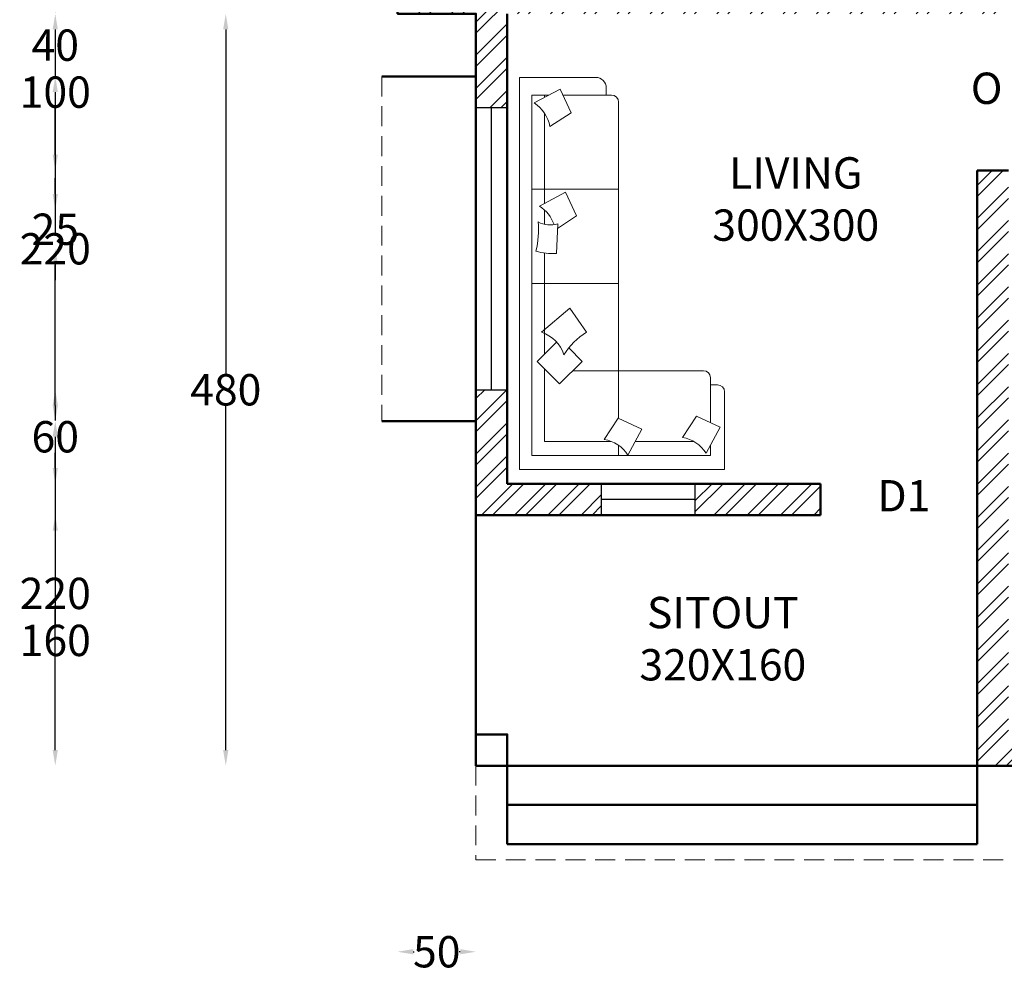
# Model space of a CAD drawing. Units: centimetres. Extents: x 10444 to 13814, y 8288 to 11191.
# Tile 2 of 9: x 10444 to 11072, y 9789 to 10397. Entities that reach past the tile are written whole.
import ezdxf

# ---------------------------------------------------------------- set-up
doc = ezdxf.new("R2010")
doc.units = ezdxf.units.CM
doc.header["$MEASUREMENT"] = 0
doc.linetypes.add('DASHED', pattern=[19.05, 12.7, -6.35])
for name, color, linetype, lineweight in [('A-ANNO-DIMS', 2, 'Continuous', 18), ('A-ANNO-TEXT', 7, 'Continuous', 25), ('A-AREA-IDEN', 3, 'Continuous', 25), ('A-FURN', 8, 'Continuous', 18), ('A-GLAZ', 4, 'Continuous', 25), ('A-ROOF-OVHD', 6, 'DASHED', 18), ('A-WALL', 7, 'Continuous', 50), ('A-WALL-PATT', 8, 'Continuous', 13)]:
    doc.layers.add(name, color=color, linetype=linetype, lineweight=lineweight)
doc.styles.get("Standard").update_dxf_attribs({"font": 'arial.ttf'})
doc.dimstyles.get("Standard").update_dxf_attribs({"dimtxt": 20, "dimasz": 10, "dimexe": 0.18, "dimexo": 0.0625, "dimgap": 0.09, "dimtad": 0, "dimtih": 1, "dimtoh": 1, "dimdec": 0, "dimzin": 0, "dimdsep": 46, "dimtxsty": 'Standard', "dimcen": 0.09, "dimse1": 1, "dimse2": 1, "dimadec": 0, "dimazin": 0, "dimtfac": 1, "dimtdec": 0, "dimtofl": 0, "dimtmove": 0, "dimatfit": 3, "dimfxl": 1, "dimtolj": 1, "dimtzin": 0, "dimarcsym": 0})

# ---------------------------------------------------------------- blocks, each defined once
blk = doc.blocks.new('s')
at = {"color": 0, "linetype": 'ByBlock'}
for p, q in [((3171.01, 851.61), (3219.52, 851.61)), ((3219.52, 851.61), (3219.52, 601.19)), ((3164.24, 840.33), (3164.24, 844.84)), ((3186.7, 829.06), (3193.66, 844.18)), ((3193.66, 844.18), (3210.33, 835.29)), ((3160.86, 840.33), (3164.24, 840.33)), ((3191.89, 840.33), (3164.24, 840.33)), ((3211.62, 840.33), (3200.88, 840.33)), ((3203.72, 840.33), (3203.72, 838.81)), ((3211.62, 610.22), (3211.62, 840.33)), ((3156.35, 633.89), (3156.35, 835.82)), ((3200.22, 820.17), (3186.7, 829.06)), ((3203.72, 828.87), (3203.72, 771.08)), ((3156.35, 780.17), (3211.62, 780.17)), ((3183.2, 763.2), (3190.16, 778.32)), ((3190.16, 778.32), (3206.83, 769.43)), ((3203.72, 767.07), (3203.72, 757.81)), ((3195.32, 755.23), (3183.2, 763.2)), ((3196, 739.19), (3195.19, 758.2)), ((3203.72, 739.46), (3203.72, 674.86)), ((3156.35, 720.01), (3211.62, 720.01)), ((3187.42, 704.35), (3176.86, 688.89)), ((3205.58, 688.89), (3187.42, 704.35)), ((3188.17, 678.84), (3179.6, 670.27)), ((3208.31, 670.27), (3195.94, 682.65)), ((3179.6, 670.27), (3193.96, 655.92)), ((3193.96, 655.92), (3208.31, 670.27)), ((3102.21, 664.36), (3156.35, 664.36)), ((3156.35, 633.89), (3156.35, 664.36)), ((3156.35, 664.36), (3185.51, 664.36)), ((3203.72, 665.68), (3203.72, 619.24)), ((3093.18, 655.34), (3097.69, 655.34)), ((3097.69, 631.14), (3097.69, 659.85)), ((3088.67, 601.19), (3088.67, 650.82)), ((3106.72, 635.3), (3091.6, 628.33)), ((3115.61, 621.77), (3106.72, 635.3)), ((3156.62, 634.01), (3141.5, 627.05)), ((3165.51, 620.48), (3156.62, 634.01)), ((3091.6, 628.33), (3100.49, 611.67)), ((3141.5, 627.05), (3150.39, 610.38)), ((3097.69, 610.22), (3097.69, 616.92)), ((3145.66, 619.24), (3108.48, 619.24)), ((3156.35, 610.22), (3156.35, 616.67)), ((3156.35, 610.22), (3156.35, 616.67)), ((3203.72, 619.24), (3161.09, 619.24)), ((3156.35, 610.22), (3097.69, 610.22)), ((3211.62, 610.22), (3156.35, 610.22)), ((3156.35, 601.19), (3088.67, 601.19)), ((3219.52, 601.19), (3156.35, 601.19))]:
    blk.add_line(p, q, dxfattribs=at)
for centre, radius, start, end in [((3171.01, 844.84), 6.77, 90, 180), ((3160.86, 835.82), 4.51, 90, 180), ((3222.32, 816.34), 22.43, 122.33007, 170.15704), ((3218.82, 750.48), 22.43, 122.33007, 161.50567), ((3200.11, 772.36), 14.99, 250.8325, 299.92347), ((3265.72, 754.9), 58.3, 175.59898, 194.04019), ((3198.69, 772.83), 33.74, 265.41548, 288.06974), ((3153.12, 650.79), 44.89, 31.93011, 58.06989), ((3212.54, 667.58), 22.42, 108.07851, 161.92149), ((3102.21, 659.85), 4.51, 90, 180), ((3093.18, 650.82), 4.51, 90, 180), ((3119.44, 599.68), 22.43, 99.84296, 147.66993), ((3169.34, 598.39), 22.43, 99.84296, 147.66993)]:
    blk.add_arc(centre, radius, start, end, dxfattribs=at)
blk = doc.blocks.new('*D12')
at = {"layer": 'A-ANNO-DIMS', "color": 0, "lineweight": -2, "transparency": 16777216}
for p, q in [((10575.11, 10390.63), (10575.11, 10170.94)), ((10575.11, 9930.63), (10575.11, 10150.33))]:
    blk.add_line(p, q, dxfattribs=at)
at = {"layer": 'A-ANNO-DIMS', "color": 0, "transparency": 16777216}
for points in [[(10573.44, 10390.63), (10576.77, 10390.63), (10575.11, 10400.63)], [(10573.44, 9930.63), (10576.77, 9930.63), (10575.11, 9920.63)]]:
    blk.add_solid(points, dxfattribs=at)
at = {"layer": 'Defpoints', "color": 0, "transparency": 16777216}
for p in [(10734.79, 10400.63), (10575.11, 9920.63), (10734.79, 9920.63)]:
    blk.add_point(p, dxfattribs=at)
at = {"layer": 'A-ANNO-DIMS', "color": 0, "transparency": 16777216, "insert": (10575.11, 10160.63), "char_height": 20, "attachment_point": 5}
blk.add_mtext('\\A1;480', dxfattribs=at)
blk = doc.blocks.new('*D13')
at = {"layer": 'A-ANNO-DIMS', "color": 0, "lineweight": -2, "transparency": 16777216}
for p, q in [((10694.79, 9801.88), (10695.41, 9801.88)), ((10724.79, 9801.88), (10724.17, 9801.88))]:
    blk.add_line(p, q, dxfattribs=at)
at = {"layer": 'A-ANNO-DIMS', "color": 0, "transparency": 16777216}
for points in [[(10694.79, 9803.55), (10694.79, 9800.21), (10684.79, 9801.88)], [(10724.79, 9803.55), (10724.79, 9800.21), (10734.79, 9801.88)]]:
    blk.add_solid(points, dxfattribs=at)
at = {"layer": 'Defpoints', "color": 0, "transparency": 16777216}
for p in [(10684.79, 10400.63), (10734.79, 10400.63), (10684.79, 9801.88)]:
    blk.add_point(p, dxfattribs=at)
at = {"layer": 'A-ANNO-DIMS', "color": 0, "transparency": 16777216, "insert": (10709.79, 9801.88), "char_height": 20, "attachment_point": 5}
blk.add_mtext('\\A1;50', dxfattribs=at)
blk = doc.blocks.new('WIN-1800')
blk.add_line((0, 10), (180, 10))
blk.add_lwpolyline([(0, 0), (180, 0), (180, 20), (0, 20)], close=True)
blk = doc.blocks.new('WIN-600')
blk.add_line((60, 10), (0, 10))
blk.add_lwpolyline([(0, 0), (60, 0), (60, 20), (0, 20)], close=True)
blk = doc.blocks.new('*D63')
at = {"layer": 'A-ANNO-DIMS', "color": 0, "lineweight": -2, "transparency": 16777216}
for p, q in [((10466.29, 10410.63), (10466.29, 10420.63)), ((10466.29, 10350.63), (10466.29, 10340.63))]:
    blk.add_line(p, q, dxfattribs=at)
at = {"layer": 'A-ANNO-DIMS', "color": 0, "transparency": 16777216}
for points in [[(10464.62, 10410.63), (10467.95, 10410.63), (10466.29, 10400.63)], [(10464.62, 10350.63), (10467.95, 10350.63), (10466.29, 10360.63)]]:
    blk.add_solid(points, dxfattribs=at)
at = {"layer": 'Defpoints', "color": 0, "transparency": 16777216}
for p in [(10684.79, 10400.63), (10466.29, 10360.63), (10674.79, 10360.63)]:
    blk.add_point(p, dxfattribs=at)
at = {"layer": 'A-ANNO-DIMS', "color": 0, "transparency": 16777216, "insert": (10466.29, 10380.63), "char_height": 20, "attachment_point": 5}
blk.add_mtext('\\A1;40', dxfattribs=at)
blk = doc.blocks.new('*D64')
at = {"layer": 'A-ANNO-DIMS', "color": 0, "lineweight": -2, "transparency": 16777216}
for p, q in [((10466.29, 10350.63), (10466.29, 10260.94)), ((10466.29, 10150.63), (10466.29, 10240.33))]:
    blk.add_line(p, q, dxfattribs=at)
at = {"layer": 'A-ANNO-DIMS', "color": 0, "transparency": 16777216}
for points in [[(10464.62, 10350.63), (10467.95, 10350.63), (10466.29, 10360.63)], [(10464.62, 10150.63), (10467.95, 10150.63), (10466.29, 10140.63)]]:
    blk.add_solid(points, dxfattribs=at)
at = {"layer": 'Defpoints', "color": 0, "transparency": 16777216}
for p in [(10674.79, 10360.63), (10466.29, 10140.63), (10674.79, 10140.63)]:
    blk.add_point(p, dxfattribs=at)
at = {"layer": 'A-ANNO-DIMS', "color": 0, "transparency": 16777216, "insert": (10466.29, 10250.63), "char_height": 20, "attachment_point": 5}
blk.add_mtext('\\A1;220', dxfattribs=at)
blk = doc.blocks.new('*D65')
at = {"layer": 'A-ANNO-DIMS', "color": 0, "lineweight": -2, "transparency": 16777216}
for p, q in [((10466.29, 10130.63), (10466.29, 10040.94)), ((10466.29, 9930.63), (10466.29, 10020.33))]:
    blk.add_line(p, q, dxfattribs=at)
at = {"layer": 'A-ANNO-DIMS', "color": 0, "transparency": 16777216}
for points in [[(10464.62, 10130.63), (10467.95, 10130.63), (10466.29, 10140.63)], [(10464.62, 9930.63), (10467.95, 9930.63), (10466.29, 9920.63)]]:
    blk.add_solid(points, dxfattribs=at)
at = {"layer": 'Defpoints', "color": 0, "transparency": 16777216}
for p in [(10674.79, 10140.63), (10466.29, 9920.63), (10734.79, 9920.63)]:
    blk.add_point(p, dxfattribs=at)
at = {"layer": 'A-ANNO-DIMS', "color": 0, "transparency": 16777216, "insert": (10466.29, 10030.63), "char_height": 20, "attachment_point": 5}
blk.add_mtext('\\A1;220', dxfattribs=at)
blk = doc.blocks.new('*D76')
at = {"layer": 'A-ANNO-DIMS', "color": 0, "lineweight": -2, "transparency": 16777216}
for p, q in [((10466.29, 10390.63), (10466.29, 10360.94)), ((10466.29, 10310.63), (10466.29, 10340.33))]:
    blk.add_line(p, q, dxfattribs=at)
at = {"layer": 'A-ANNO-DIMS', "color": 0, "transparency": 16777216}
for points in [[(10464.62, 10390.63), (10467.95, 10390.63), (10466.29, 10400.63)], [(10464.62, 10310.63), (10467.95, 10310.63), (10466.29, 10300.63)]]:
    blk.add_solid(points, dxfattribs=at)
at = {"layer": 'Defpoints', "color": 0, "transparency": 16777216}
for p in [(10466.29, 10400.63), (11114.79, 10400.63), (11054.79, 10300.63)]:
    blk.add_point(p, dxfattribs=at)
at = {"layer": 'A-ANNO-DIMS', "color": 0, "transparency": 16777216, "insert": (10466.29, 10350.63), "char_height": 20, "attachment_point": 5}
blk.add_mtext('\\A1;100', dxfattribs=at)
blk = doc.blocks.new('*D78')
at = {"layer": 'A-ANNO-DIMS', "color": 0, "lineweight": -2, "transparency": 16777216}
for p, q in [((10684.79, 11178), (10690.35, 11178)), ((10724.79, 11178), (10719.22, 11178))]:
    blk.add_line(p, q, dxfattribs=at)
at = {"layer": 'A-ANNO-DIMS', "color": 0, "transparency": 16777216}
for points in [[(10684.79, 11179.67), (10684.79, 11176.33), (10674.79, 11178)], [(10724.79, 11179.67), (10724.79, 11176.33), (10734.79, 11178)]]:
    blk.add_solid(points, dxfattribs=at)
at = {"layer": 'Defpoints', "color": 0, "transparency": 16777216}
for p in [(10734.79, 11178), (10674.79, 10360.63), (10734.79, 10360.63)]:
    blk.add_point(p, dxfattribs=at)
at = {"layer": 'A-ANNO-DIMS', "color": 0, "transparency": 16777216, "insert": (10704.79, 11178), "char_height": 20, "attachment_point": 5}
blk.add_mtext('\\A1;60', dxfattribs=at)
blk = doc.blocks.new('*D79')
at = {"layer": 'A-ANNO-DIMS', "color": 0, "lineweight": -2, "transparency": 16777216}
for p, q in [((10466.29, 10150.63), (10466.29, 10140.94)), ((10466.29, 10110.63), (10466.29, 10120.33))]:
    blk.add_line(p, q, dxfattribs=at)
at = {"layer": 'A-ANNO-DIMS', "color": 0, "transparency": 16777216}
for points in [[(10464.62, 10150.63), (10467.95, 10150.63), (10466.29, 10160.63)], [(10464.62, 10110.63), (10467.95, 10110.63), (10466.29, 10100.63)]]:
    blk.add_solid(points, dxfattribs=at)
at = {"layer": 'Defpoints', "color": 0, "transparency": 16777216}
for p in [(10466.29, 10160.63), (10754.79, 10160.63), (10754.79, 10100.63)]:
    blk.add_point(p, dxfattribs=at)
at = {"layer": 'A-ANNO-DIMS', "color": 0, "transparency": 16777216, "insert": (10466.29, 10130.63), "char_height": 20, "attachment_point": 5}
blk.add_mtext('\\A1;60', dxfattribs=at)
blk = doc.blocks.new('*D81')
at = {"layer": 'A-ANNO-DIMS', "color": 0, "lineweight": -2, "transparency": 16777216}
for p, q in [((10466.29, 10070.63), (10466.29, 10010.94)), ((10466.29, 9930.63), (10466.29, 9990.33))]:
    blk.add_line(p, q, dxfattribs=at)
at = {"layer": 'A-ANNO-DIMS', "color": 0, "transparency": 16777216}
for points in [[(10464.62, 10070.63), (10467.95, 10070.63), (10466.29, 10080.63)], [(10464.62, 9930.63), (10467.95, 9930.63), (10466.29, 9920.63)]]:
    blk.add_solid(points, dxfattribs=at)
at = {"layer": 'Defpoints', "color": 0, "transparency": 16777216}
for p in [(10466.29, 10080.63), (11664.79, 10080.63), (11664.79, 9920.63)]:
    blk.add_point(p, dxfattribs=at)
at = {"layer": 'A-ANNO-DIMS', "color": 0, "transparency": 16777216, "insert": (10466.29, 10000.63), "char_height": 20, "attachment_point": 5}
blk.add_mtext('\\A1;160', dxfattribs=at)
blk = doc.blocks.new('*D85')
at = {"layer": 'A-ANNO-DIMS', "color": 0, "lineweight": -2, "transparency": 16777216}
for p, q in [((10466.29, 10285.63), (10466.29, 10295.63)), ((10466.29, 10240.63), (10466.29, 10230.63))]:
    blk.add_line(p, q, dxfattribs=at)
at = {"layer": 'A-ANNO-DIMS', "color": 0, "transparency": 16777216}
for points in [[(10464.62, 10285.63), (10467.95, 10285.63), (10466.29, 10275.63)], [(10464.62, 10240.63), (10467.95, 10240.63), (10466.29, 10250.63)]]:
    blk.add_solid(points, dxfattribs=at)
at = {"layer": 'Defpoints', "color": 0, "transparency": 16777216}
for p in [(11164.79, 10275.63), (10466.29, 10250.63), (11164.79, 10250.63)]:
    blk.add_point(p, dxfattribs=at)
at = {"layer": 'A-ANNO-DIMS', "color": 0, "transparency": 16777216, "insert": (10466.29, 10263.13), "char_height": 20, "attachment_point": 5}
blk.add_mtext('\\A1;25', dxfattribs=at)

msp = doc.modelspace()

# ---------------------------------------------------------------- hatches: boundary and pattern name
at = {"layer": 'A-WALL-PATT'}
h = msp.add_hatch(dxfattribs=at)
h.set_pattern_fill('ANSI32', color=256, scale=40)
h.paths.add_polyline_path([(10809.7881, 10800.6336), (10684.7881, 10800.6336), (10684.7881, 10690.6336), (10704.7881, 10690.6336), (10704.7881, 10726.41), (10704.7881, 10780.6336), (10809.7881, 10780.6336)])
h.paths.add_polyline_path([(11154.7881, 10800.6336), (10989.7881, 10800.6336), (10989.7881, 10780.6336), (11114.7881, 10780.6336), (11154.7881, 10780.6336)])
h.paths.add_polyline_path([(11354.7881, 10800.6336), (11214.7881, 10800.6336), (11214.7881, 10780.6336), (11254.7881, 10780.6336), (11254.7881, 10582.9925, -0.00499308), (11254.7881, 10581.0383), (11254.7881, 10571.0719, -0.26947312), (11256.5873, 10571.9821), (11256.5873, 10568.3227), (11256.5873, 10564.4272, -0.26947312), (11254.7881, 10565.3375), (11254.7881, 10530.6336), (11196.6819, 10530.6336), (11196.6819, 10510.6336), (11254.7881, 10510.6336), (11254.7881, 10400.6336), (11274.7881, 10400.6336), (11274.7881, 10420.6336), (11274.7881, 10780.6336), (11354.7881, 10780.6336)])
h.paths.add_polyline_path([(10704.7881, 10510.6336), (10684.7881, 10510.6336), (10684.7881, 10400.6336), (10734.7881, 10400.6336), (10734.7881, 10340.6336), (10754.7881, 10340.6336), (10754.7881, 10400.6336), (11114.7881, 10400.6336), (11114.7881, 10420.6336), (10704.7881, 10420.6336)])
h.paths.add_polyline_path([(11794.7881, 10420.6336), (11364.7881, 10420.6336), (11364.7881, 10400.6336), (11644.7881, 10400.6336), (11644.7881, 10260.6336), (11664.7881, 10260.6336), (11664.7881, 10400.6336), (11794.7881, 10400.6336)])
h.paths.add_polyline_path([(11594.7881, 10670.6336), (11594.7881, 10708.9482, -0.26828041), (11592.9938, 10708.0455), (11592.9938, 10711.9409), (11592.9938, 10715.6003, -0.26828041), (11594.7881, 10714.6976), (11594.7881, 10780.6336), (11654.7881, 10780.6336), (11654.7881, 10800.6336), (11494.7881, 10800.6336), (11494.7881, 10780.6336), (11574.7881, 10780.6336), (11574.7881, 10510.6336), (11594.7881, 10510.6336)])
h.paths.add_polyline_path([(11794.7881, 10800.6336), (11714.7881, 10800.6336), (11714.7881, 10780.6336), (11774.7881, 10780.6336), (11774.7881, 10750.6336), (11794.7881, 10750.6336)])
h.paths.add_polyline_path([(11794.7881, 10670.6336), (11674.7881, 10670.6336), (11674.7881, 10650.6336), (11794.7881, 10650.6336)])
h.paths.add_polyline_path([(11664.7881, 10080.6336), (11644.7881, 10080.6336), (11644.7881, 9940.6336), (11549.7881, 9940.6336), (11549.7881, 9920.6336), (11664.7881, 9920.6336)])
h.paths.add_polyline_path([(11369.7881, 9940.6336), (11274.7881, 9940.6336), (11274.7881, 10300.6336), (11254.7881, 10300.6336), (11254.7881, 9940.6336), (11234.7881, 9940.6336), (11234.7881, 9920.6336), (11369.7881, 9920.6336)])
h.paths.add_polyline_path([(11094.7881, 9940.6336), (11074.7881, 9940.6336), (11074.7881, 10300.6336), (11054.7881, 10300.6336), (11054.7881, 10080.6336), (11054.7881, 9920.6336), (11094.7881, 9920.6336)])
h.paths.add_polyline_path([(11134.7881, 9940.6336), (11114.7881, 9940.6336), (11114.7881, 9920.6336), (11134.7881, 9920.6336)])
h.paths.add_polyline_path([(11174.7881, 9940.6336), (11154.7881, 9940.6336), (11154.7881, 9920.6336), (11174.7881, 9920.6336)])
h.paths.add_polyline_path([(11214.7881, 9940.6336), (11196.6819, 9940.6336), (11196.6819, 9920.6336), (11214.7881, 9920.6336)])
h.paths.add_polyline_path([(10954.7881, 10100.6336), (10874.7881, 10100.6336), (10874.7881, 10080.6336), (10954.7881, 10080.6336)])
h.paths.add_polyline_path([(10814.7881, 10100.6336), (10754.7881, 10100.6336), (10754.7881, 10160.6336), (10734.7881, 10160.6336), (10734.7881, 10080.6336), (10814.7881, 10080.6336)])
h.paths.add_polyline_path([(11255.1494, 10331.8339), (11286.882, 10331.8339), (11286.882, 10373.0481), (11255.1494, 10373.0481)], flags=9)
h.paths.add_polyline_path([(11607.8445, 10630.7128), (11653.5607, 10630.7128), (11653.5607, 10671.927), (11607.8445, 10671.927)], flags=25)
h.paths.add_polyline_path([(11746.8445, 10447.0791), (11792.5607, 10447.0791), (11792.5607, 10488.2933), (11746.8445, 10488.2933)], flags=9)
h.paths.add_polyline_path([(11296.8445, 10388.5791), (11342.5607, 10388.5791), (11342.5607, 10429.7933), (11296.8445, 10429.7933)], flags=9)
h.paths.add_polyline_path([(11376.6416, 10156.0222), (11521.6757, 10156.0222), (11521.6757, 10230.6515), (11376.6416, 10230.6515)], flags=9)
h.paths.add_polyline_path([(11437.3982, 10313.4478), (11545.1881, 10313.4478), (11545.1881, 10354.662), (11437.3982, 10354.662)], flags=25)
h.paths.add_polyline_path([(11655.4027, 10682.0329), (11777.2718, 10682.0329), (11777.2718, 10756.6623), (11655.4027, 10756.6623)], flags=9)
h.paths.add_polyline_path([(11636.2626, 10500.0811), (11758.1316, 10500.0811), (11758.1316, 10574.7105), (11636.2626, 10574.7105)], flags=9)
h.paths.add_polyline_path([(11336.6251, 10562.3234), (11469.2581, 10562.3234), (11469.2581, 10636.9528), (11336.6251, 10636.9528)], flags=9)

# ---------------------------------------------------------------- linework, layer by layer
at = {"layer": 'A-ROOF-OVHD'}
for p, q in [((10674.7881, 10360.6336), (10674.7881, 10140.6336)), ((10734.7881, 9920.6336), (10734.7881, 9860.6336)), ((10734.7881, 9860.6336), (11074.7881, 9860.6336))]:
    msp.add_line(p, q, dxfattribs=at)
at = {"layer": 'A-WALL'}
for p, q in [((10734.7881, 10400.6336), (10734.7881, 9940.6336)), ((10754.7881, 10400.6336), (10754.7881, 10100.6336)), ((10734.7881, 10360.6336), (10674.7881, 10360.6336)), ((10734.7881, 10340.6336), (10734.7881, 10360.6336)), ((11054.7881, 10300.6336), (11054.7881, 10080.6336)), ((11074.7881, 10300.6336), (11054.7881, 10300.6336)), ((10734.7881, 10160.6336), (10734.7881, 10140.6336)), ((10734.7881, 10140.6336), (10674.7881, 10140.6336)), ((10754.7881, 10100.6336), (10954.7881, 10100.6336)), ((10954.7881, 10100.6336), (10954.7881, 10080.6336)), ((10734.7881, 10080.6336), (10954.7881, 10080.6336)), ((11054.7881, 10080.6336), (11054.7881, 9920.6336)), ((10754.7881, 9920.6336), (11664.7881, 9920.6336)), ((10754.7881, 9870.6336), (10754.7881, 9920.6336)), ((11054.7881, 9920.6336), (11054.7881, 9870.6336)), ((10754.7881, 9895.6336), (11054.7881, 9895.6336)), ((10754.7881, 9870.6336), (11054.7881, 9870.6336))]:
    msp.add_line(p, q, dxfattribs=at)
msp.add_lwpolyline([(10734.7881, 9920.6336), (11664.7881, 9920.6336), (11664.7881, 10400.6336), (11794.7881, 10400.6336), (11794.7881, 10800.6336), (10684.7881, 10800.6336), (10684.7881, 10400.6336), (10734.7881, 10400.6336), (10734.7881, 9920.6336)], dxfattribs=at)
msp.add_lwpolyline([(10734.7881, 9920.6336), (10754.7881, 9920.6336), (10754.7881, 9940.6336), (10734.7881, 9940.6336)], close=True, dxfattribs=at)

# ---------------------------------------------------------------- block references
at = {"layer": 'A-FURN', "xscale": -1}
msp.add_blockref('s', (13982.2009, 9508.4652), dxfattribs=at)
at = {"layer": 'A-GLAZ', "rotation": 90.00000000000101}
msp.add_blockref('WIN-1800', (10754.7877, 10160.6335), dxfattribs=at)
at = {"layer": 'A-GLAZ'}
msp.add_blockref('WIN-600', (10814.788, 10080.634), dxfattribs=at)

# ---------------------------------------------------------------- texts
at = {"layer": 'A-ANNO-TEXT', "char_height": 20, "attachment_point": 1}
for s, insert in [('O', (11050.6664, 10363.1095)), ('D1', (10991, 10103))]:
    msp.add_mtext_dynamic_manual_height_columns(s, width=668.5, gutter_width=1, heights=[0], dxfattribs=dict(at, insert=insert))
at = {"layer": 'A-AREA-IDEN', "char_height": 20, "attachment_point": 1}
for s, insert in [('\\pxqc;LIVING\\P300X300', (10864.6044, 10309.0931)), ('\\pxqc;SITOUT\\P320X160', (10818.0598, 10028.404))]:
    msp.add_mtext_dynamic_manual_height_columns(s, width=148.64167, gutter_width=1, heights=[0], dxfattribs=dict(at, insert=insert))

# ---------------------------------------------------------------- dimensions: what is measured, and where the dimension line sits
at = {"layer": 'A-ANNO-DIMS'}
dim = msp.add_linear_dim(base=(10734.7881, 11178), p1=(10674.7881, 10360.6336), p2=(10734.7881, 10360.6336), dimstyle='Standard', override={"dimdec": 0, "dimlfac": 1, "dimrnd": 0, "dimzin": 0, "dimdsep": 46, "dimlunit": 2}, dxfattribs=at)
dim.commit()
dim.dimension.update_dxf_attribs({"geometry": '*D78', "text_midpoint": (10704.7881, 11178)})
for base, p1, p2, picture, middle in [((10466.2881, 10360.6336), (10684.7881, 10400.6336), (10674.7881, 10360.6336), '*D63', (10466.2881, 10380.6336)), ((10466.2881, 10400.6336), (11054.7881, 10300.6336), (11114.7881, 10400.6336), '*D76', (10466.2881, 10350.6336)), ((10466.2881, 10140.6336), (10674.7881, 10360.6336), (10674.7881, 10140.6336), '*D64', (10466.2881, 10250.6336)), ((10466.2881, 10250.6336), (11164.7881, 10275.6336), (11164.7881, 10250.6336), '*D85', (10466.2881, 10263.1336)), ((10466.2881, 10160.6336), (10754.7881, 10100.6336), (10754.7881, 10160.6336), '*D79', (10466.2881, 10130.6336)), ((10466.2881, 9920.6336), (10674.7881, 10140.6336), (10734.7881, 9920.6336), '*D65', (10466.2881, 10030.6336)), ((10466.2881, 10080.6336), (11664.7881, 9920.6336), (11664.7881, 10080.6336), '*D81', (10466.2881, 10000.6336))]:
    dim = msp.add_linear_dim(base=base, p1=p1, p2=p2, angle=90, dimstyle='Standard', override={"dimdec": 0, "dimlfac": 1, "dimrnd": 0, "dimzin": 0, "dimdsep": 46, "dimlunit": 2}, dxfattribs=at)
    dim.commit()
    dim.dimension.update_dxf_attribs({"geometry": picture, "text_midpoint": middle})
for p2, distance, picture, middle in [((10734.7881, 9920.6336), -159.6819, '*D12', (10575.1062, 10160.6336)), ((10684.7881, 10400.6336), 598.7533, '*D13', (10709.7881, 9801.8804))]:
    dim = msp.add_aligned_dim(p1=(10734.7881, 10400.6336), p2=p2, distance=distance, dimstyle='Standard', override={"dimclrd": 0, "dimclre": 0, "dimclrt": 0}, dxfattribs=at)
    dim.commit()
    dim.dimension.update_dxf_attribs({"geometry": picture, "text_midpoint": middle})

doc.saveas('drawing.dxf')
